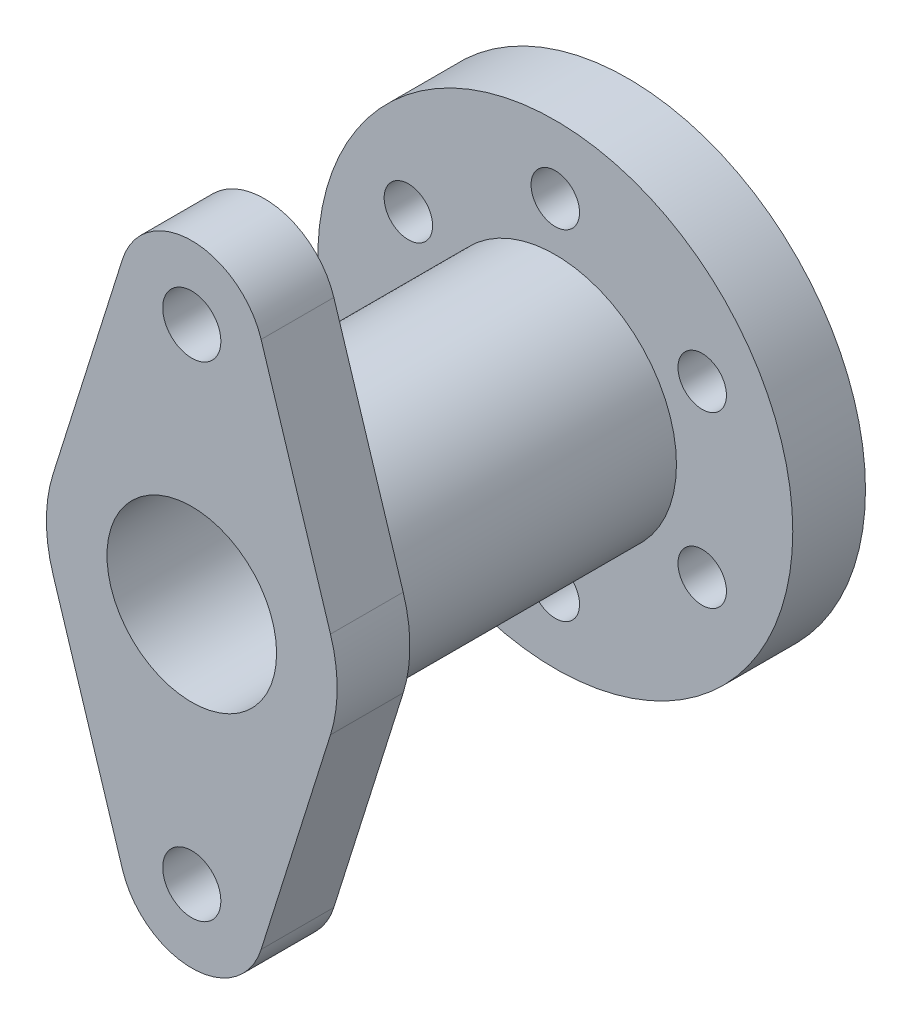
ISO-10303-21;
HEADER;
FILE_DESCRIPTION(('STEP AP214'),'2;1');
FILE_NAME('part.step','',(''),(''),'','','');
FILE_SCHEMA(('AUTOMOTIVE_DESIGN { 1 0 10303 214 1 1 1 1 }'));
ENDSEC;
DATA;
#1=APPLICATION_CONTEXT('core data for automotive mechanical design processes');
#2=APPLICATION_PROTOCOL_DEFINITION('international standard','automotive_design',2000,#1);
#3=PRODUCT_CONTEXT('',#1,'mechanical');
#4=PRODUCT('Part','Part','',(#3));
#5=PRODUCT_RELATED_PRODUCT_CATEGORY('part','',(#4));
#6=PRODUCT_DEFINITION_FORMATION('','',#4);
#7=PRODUCT_DEFINITION_CONTEXT('part definition',#1,'design');
#8=PRODUCT_DEFINITION('design','',#6,#7);
#9=PRODUCT_DEFINITION_SHAPE('','',#8);
#10=(LENGTH_UNIT() NAMED_UNIT(*) SI_UNIT(.MILLI.,.METRE.));
#11=(NAMED_UNIT(*) PLANE_ANGLE_UNIT() SI_UNIT($,.RADIAN.));
#12=(NAMED_UNIT(*) SI_UNIT($,.STERADIAN.) SOLID_ANGLE_UNIT());
#13=UNCERTAINTY_MEASURE_WITH_UNIT(LENGTH_MEASURE(1.E-05),#10,'distance_accuracy_value','');
#14=(GEOMETRIC_REPRESENTATION_CONTEXT(3) GLOBAL_UNCERTAINTY_ASSIGNED_CONTEXT((#13)) GLOBAL_UNIT_ASSIGNED_CONTEXT((#10,
#11,#12)) REPRESENTATION_CONTEXT('',''));
#15=CARTESIAN_POINT('',(0.,0.,0.));
#16=DIRECTION('',(0.,0.,1.));
#17=DIRECTION('',(1.,0.,0.));
#18=AXIS2_PLACEMENT_3D('',#15,#16,#17);
#19=CARTESIAN_POINT('',(0.,0.,60.));
#20=DIRECTION('',(0.,0.,1.));
#21=DIRECTION('',(1.,0.,0.));
#22=AXIS2_PLACEMENT_3D('',#19,#20,#21);
#23=PLANE('',#22);
#24=CARTESIAN_POINT('',(0.,0.,60.));
#25=DIRECTION('',(0.,0.,1.));
#26=DIRECTION('',(1.,0.,0.));
#27=AXIS2_PLACEMENT_3D('',#24,#25,#26);
#28=CIRCLE('',#27,13.);
#29=CARTESIAN_POINT('',(13.,0.,60.));
#30=VERTEX_POINT('',#29);
#31=EDGE_CURVE('E194',#30,#30,#28,.T.);
#32=ORIENTED_EDGE('',*,*,#31,.F.);
#33=EDGE_LOOP('',(#32));
#34=FACE_BOUND('',#33,.T.);
#35=CARTESIAN_POINT('',(0.,0.,60.));
#36=DIRECTION('',(0.,0.,1.));
#37=DIRECTION('',(1.,0.,0.));
#38=AXIS2_PLACEMENT_3D('',#35,#36,#37);
#39=CIRCLE('',#38,17.5);
#40=CARTESIAN_POINT('',(17.5,0.,60.));
#41=VERTEX_POINT('',#40);
#42=EDGE_CURVE('E187',#41,#41,#39,.T.);
#43=ORIENTED_EDGE('',*,*,#42,.T.);
#44=EDGE_LOOP('',(#43));
#45=FACE_BOUND('',#44,.T.);
#46=ADVANCED_FACE('F50',(#34,#45),#23,.T.);
#47=CARTESIAN_POINT('',(0.,0.,15.));
#48=DIRECTION('',(0.,0.,1.));
#49=DIRECTION('',(1.,0.,0.));
#50=AXIS2_PLACEMENT_3D('',#47,#48,#49);
#51=PLANE('',#50);
#52=CARTESIAN_POINT('',(-30.3108891324546,17.4999999999987,15.));
#53=DIRECTION('',(0.,0.,1.));
#54=DIRECTION('',(1.,0.,0.));
#55=AXIS2_PLACEMENT_3D('',#52,#53,#54);
#56=CIRCLE('',#55,5.0000000000015);
#57=CARTESIAN_POINT('',(-25.3108891324531,17.4999999999987,15.));
#58=VERTEX_POINT('',#57);
#59=EDGE_CURVE('E203',#58,#58,#56,.T.);
#60=ORIENTED_EDGE('',*,*,#59,.F.);
#61=EDGE_LOOP('',(#60));
#62=FACE_BOUND('',#61,.T.);
#63=CARTESIAN_POINT('',(2.97142069880137E-12,-35.,15.));
#64=DIRECTION('',(0.,0.,1.));
#65=DIRECTION('',(1.,0.,0.));
#66=AXIS2_PLACEMENT_3D('',#63,#64,#65);
#67=CIRCLE('',#66,5.00000000000308);
#68=CARTESIAN_POINT('',(5.00000000000605,-35.,15.));
#69=VERTEX_POINT('',#68);
#70=EDGE_CURVE('E213',#69,#69,#67,.T.);
#71=ORIENTED_EDGE('',*,*,#70,.F.);
#72=EDGE_LOOP('',(#71));
#73=FACE_BOUND('',#72,.T.);
#74=CARTESIAN_POINT('',(30.3108891324561,17.5000000000013,15.));
#75=DIRECTION('',(0.,0.,1.));
#76=DIRECTION('',(1.,0.,0.));
#77=AXIS2_PLACEMENT_3D('',#74,#75,#76);
#78=CIRCLE('',#77,5.00000000000041);
#79=CARTESIAN_POINT('',(35.3108891324565,17.5000000000013,15.));
#80=VERTEX_POINT('',#79);
#81=EDGE_CURVE('E223',#80,#80,#78,.T.);
#82=ORIENTED_EDGE('',*,*,#81,.F.);
#83=EDGE_LOOP('',(#82));
#84=FACE_BOUND('',#83,.T.);
#85=CARTESIAN_POINT('',(0.,0.,15.));
#86=DIRECTION('',(0.,0.,1.));
#87=DIRECTION('',(1.,0.,0.));
#88=AXIS2_PLACEMENT_3D('',#85,#86,#87);
#89=CIRCLE('',#88,49.);
#90=CARTESIAN_POINT('',(49.,0.,15.));
#91=VERTEX_POINT('',#90);
#92=EDGE_CURVE('E11',#91,#91,#89,.T.);
#93=ORIENTED_EDGE('',*,*,#92,.T.);
#94=EDGE_LOOP('',(#93));
#95=FACE_BOUND('',#94,.T.);
#96=CARTESIAN_POINT('',(0.,35.,15.));
#97=DIRECTION('',(0.,0.,1.));
#98=DIRECTION('',(1.,0.,0.));
#99=AXIS2_PLACEMENT_3D('',#96,#97,#98);
#100=CIRCLE('',#99,5.);
#101=CARTESIAN_POINT('',(5.,35.,15.));
#102=VERTEX_POINT('',#101);
#103=EDGE_CURVE('E233',#102,#102,#100,.T.);
#104=ORIENTED_EDGE('',*,*,#103,.F.);
#105=EDGE_LOOP('',(#104));
#106=FACE_BOUND('',#105,.T.);
#107=CARTESIAN_POINT('',(30.3108891324576,-17.4999999999987,15.));
#108=DIRECTION('',(0.,0.,1.));
#109=DIRECTION('',(1.,0.,0.));
#110=AXIS2_PLACEMENT_3D('',#107,#108,#109);
#111=CIRCLE('',#110,5.00000000000192);
#112=CARTESIAN_POINT('',(35.3108891324595,-17.4999999999987,15.));
#113=VERTEX_POINT('',#112);
#114=EDGE_CURVE('E218',#113,#113,#111,.T.);
#115=ORIENTED_EDGE('',*,*,#114,.F.);
#116=EDGE_LOOP('',(#115));
#117=FACE_BOUND('',#116,.T.);
#118=CARTESIAN_POINT('',(-30.3108891324531,-17.5000000000013,15.));
#119=DIRECTION('',(0.,0.,1.));
#120=DIRECTION('',(1.,0.,0.));
#121=AXIS2_PLACEMENT_3D('',#118,#119,#120);
#122=CIRCLE('',#121,5.00000000000282);
#123=CARTESIAN_POINT('',(-25.3108891324503,-17.5000000000013,15.));
#124=VERTEX_POINT('',#123);
#125=EDGE_CURVE('E210',#124,#124,#122,.T.);
#126=ORIENTED_EDGE('',*,*,#125,.F.);
#127=EDGE_LOOP('',(#126));
#128=FACE_BOUND('',#127,.T.);
#129=CARTESIAN_POINT('',(0.,0.,15.));
#130=DIRECTION('',(0.,0.,1.));
#131=DIRECTION('',(1.,0.,0.));
#132=AXIS2_PLACEMENT_3D('',#129,#130,#131);
#133=CIRCLE('',#132,25.);
#134=CARTESIAN_POINT('',(-25.,0.,15.));
#135=VERTEX_POINT('',#134);
#136=EDGE_CURVE('E197',#135,#135,#133,.T.);
#137=ORIENTED_EDGE('',*,*,#136,.F.);
#138=EDGE_LOOP('',(#137));
#139=FACE_BOUND('',#138,.T.);
#140=ADVANCED_FACE('F248',(#62,#73,#84,#95,#106,#117,#128,#139),#51,.T.);
#141=CARTESIAN_POINT('',(0.,0.,0.));
#142=DIRECTION('',(0.,0.,1.));
#143=DIRECTION('',(1.,0.,0.));
#144=AXIS2_PLACEMENT_3D('',#141,#142,#143);
#145=PLANE('',#144);
#146=CARTESIAN_POINT('',(0.,0.,0.));
#147=DIRECTION('',(0.,0.,1.));
#148=DIRECTION('',(1.,0.,0.));
#149=AXIS2_PLACEMENT_3D('',#146,#147,#148);
#150=CIRCLE('',#149,49.);
#151=CARTESIAN_POINT('',(49.,0.,0.));
#152=VERTEX_POINT('',#151);
#153=EDGE_CURVE('E51',#152,#152,#150,.T.);
#154=ORIENTED_EDGE('',*,*,#153,.F.);
#155=EDGE_LOOP('',(#154));
#156=FACE_BOUND('',#155,.T.);
#157=CARTESIAN_POINT('',(0.,0.,0.));
#158=DIRECTION('',(0.,0.,1.));
#159=DIRECTION('',(1.,0.,0.));
#160=AXIS2_PLACEMENT_3D('',#157,#158,#159);
#161=CIRCLE('',#160,13.);
#162=CARTESIAN_POINT('',(13.,0.,0.));
#163=VERTEX_POINT('',#162);
#164=EDGE_CURVE('E234',#163,#163,#161,.T.);
#165=ORIENTED_EDGE('',*,*,#164,.T.);
#166=EDGE_LOOP('',(#165));
#167=FACE_BOUND('',#166,.T.);
#168=CARTESIAN_POINT('',(0.,35.,0.));
#169=DIRECTION('',(0.,0.,1.));
#170=DIRECTION('',(1.,0.,0.));
#171=AXIS2_PLACEMENT_3D('',#168,#169,#170);
#172=CIRCLE('',#171,5.);
#173=CARTESIAN_POINT('',(5.,35.,0.));
#174=VERTEX_POINT('',#173);
#175=EDGE_CURVE('E227',#174,#174,#172,.T.);
#176=ORIENTED_EDGE('',*,*,#175,.T.);
#177=EDGE_LOOP('',(#176));
#178=FACE_BOUND('',#177,.T.);
#179=CARTESIAN_POINT('',(30.3108891324561,17.5000000000013,0.));
#180=DIRECTION('',(0.,0.,1.));
#181=DIRECTION('',(1.,0.,0.));
#182=AXIS2_PLACEMENT_3D('',#179,#180,#181);
#183=CIRCLE('',#182,5.00000000000041);
#184=CARTESIAN_POINT('',(35.3108891324565,17.5000000000013,0.));
#185=VERTEX_POINT('',#184);
#186=EDGE_CURVE('E225',#185,#185,#183,.T.);
#187=ORIENTED_EDGE('',*,*,#186,.T.);
#188=EDGE_LOOP('',(#187));
#189=FACE_BOUND('',#188,.T.);
#190=CARTESIAN_POINT('',(30.3108891324576,-17.4999999999987,0.));
#191=DIRECTION('',(0.,0.,1.));
#192=DIRECTION('',(1.,0.,0.));
#193=AXIS2_PLACEMENT_3D('',#190,#191,#192);
#194=CIRCLE('',#193,5.00000000000192);
#195=CARTESIAN_POINT('',(35.3108891324595,-17.4999999999987,0.));
#196=VERTEX_POINT('',#195);
#197=EDGE_CURVE('E216',#196,#196,#194,.T.);
#198=ORIENTED_EDGE('',*,*,#197,.T.);
#199=EDGE_LOOP('',(#198));
#200=FACE_BOUND('',#199,.T.);
#201=CARTESIAN_POINT('',(2.97142069880137E-12,-35.,0.));
#202=DIRECTION('',(0.,0.,1.));
#203=DIRECTION('',(1.,0.,0.));
#204=AXIS2_PLACEMENT_3D('',#201,#202,#203);
#205=CIRCLE('',#204,5.00000000000308);
#206=CARTESIAN_POINT('',(5.00000000000605,-35.,0.));
#207=VERTEX_POINT('',#206);
#208=EDGE_CURVE('E209',#207,#207,#205,.T.);
#209=ORIENTED_EDGE('',*,*,#208,.T.);
#210=EDGE_LOOP('',(#209));
#211=FACE_BOUND('',#210,.T.);
#212=CARTESIAN_POINT('',(-30.3108891324531,-17.5000000000013,0.));
#213=DIRECTION('',(0.,0.,1.));
#214=DIRECTION('',(1.,0.,0.));
#215=AXIS2_PLACEMENT_3D('',#212,#213,#214);
#216=CIRCLE('',#215,5.00000000000282);
#217=CARTESIAN_POINT('',(-25.3108891324503,-17.5000000000013,0.));
#218=VERTEX_POINT('',#217);
#219=EDGE_CURVE('E204',#218,#218,#216,.T.);
#220=ORIENTED_EDGE('',*,*,#219,.T.);
#221=EDGE_LOOP('',(#220));
#222=FACE_BOUND('',#221,.T.);
#223=CARTESIAN_POINT('',(-30.3108891324546,17.4999999999987,0.));
#224=DIRECTION('',(0.,0.,1.));
#225=DIRECTION('',(1.,0.,0.));
#226=AXIS2_PLACEMENT_3D('',#223,#224,#225);
#227=CIRCLE('',#226,5.0000000000015);
#228=CARTESIAN_POINT('',(-25.3108891324531,17.4999999999987,0.));
#229=VERTEX_POINT('',#228);
#230=EDGE_CURVE('E199',#229,#229,#227,.T.);
#231=ORIENTED_EDGE('',*,*,#230,.T.);
#232=EDGE_LOOP('',(#231));
#233=FACE_BOUND('',#232,.T.);
#234=ADVANCED_FACE('F243',(#156,#167,#178,#189,#200,#211,#222,#233),#145,.F.);
#235=CARTESIAN_POINT('',(0.,0.,15.));
#236=DIRECTION('',(0.,0.,-1.));
#237=DIRECTION('',(-1.,0.,0.));
#238=AXIS2_PLACEMENT_3D('',#235,#236,#237);
#239=CYLINDRICAL_SURFACE('',#238,49.);
#240=ORIENTED_EDGE('',*,*,#92,.F.);
#241=EDGE_LOOP('',(#240));
#242=FACE_BOUND('',#241,.T.);
#243=ORIENTED_EDGE('',*,*,#153,.T.);
#244=EDGE_LOOP('',(#243));
#245=FACE_BOUND('',#244,.T.);
#246=ADVANCED_FACE('F47',(#242,#245),#239,.T.);
#247=CARTESIAN_POINT('',(0.,0.,15.));
#248=DIRECTION('',(0.,0.,-1.));
#249=DIRECTION('',(-1.,0.,0.));
#250=AXIS2_PLACEMENT_3D('',#247,#248,#249);
#251=CYLINDRICAL_SURFACE('',#250,13.);
#252=ORIENTED_EDGE('',*,*,#164,.F.);
#253=EDGE_LOOP('',(#252));
#254=FACE_BOUND('',#253,.T.);
#255=ORIENTED_EDGE('',*,*,#31,.T.);
#256=EDGE_LOOP('',(#255));
#257=FACE_BOUND('',#256,.T.);
#258=ADVANCED_FACE('F556',(#254,#257),#251,.F.);
#259=CARTESIAN_POINT('',(0.,35.,15.));
#260=DIRECTION('',(0.,0.,-1.));
#261=DIRECTION('',(-1.,0.,0.));
#262=AXIS2_PLACEMENT_3D('',#259,#260,#261);
#263=CYLINDRICAL_SURFACE('',#262,5.);
#264=ORIENTED_EDGE('',*,*,#103,.T.);
#265=EDGE_LOOP('',(#264));
#266=FACE_BOUND('',#265,.T.);
#267=ORIENTED_EDGE('',*,*,#175,.F.);
#268=EDGE_LOOP('',(#267));
#269=FACE_BOUND('',#268,.T.);
#270=ADVANCED_FACE('F546',(#266,#269),#263,.F.);
#271=CARTESIAN_POINT('',(30.3108891324561,17.5000000000013,15.));
#272=DIRECTION('',(0.,0.,-1.));
#273=DIRECTION('',(-1.,0.,0.));
#274=AXIS2_PLACEMENT_3D('',#271,#272,#273);
#275=CYLINDRICAL_SURFACE('',#274,5.00000000000041);
#276=ORIENTED_EDGE('',*,*,#81,.T.);
#277=EDGE_LOOP('',(#276));
#278=FACE_BOUND('',#277,.T.);
#279=ORIENTED_EDGE('',*,*,#186,.F.);
#280=EDGE_LOOP('',(#279));
#281=FACE_BOUND('',#280,.T.);
#282=ADVANCED_FACE('F536',(#278,#281),#275,.F.);
#283=CARTESIAN_POINT('',(30.3108891324576,-17.4999999999987,15.));
#284=DIRECTION('',(0.,0.,-1.));
#285=DIRECTION('',(-1.,0.,0.));
#286=AXIS2_PLACEMENT_3D('',#283,#284,#285);
#287=CYLINDRICAL_SURFACE('',#286,5.00000000000192);
#288=ORIENTED_EDGE('',*,*,#114,.T.);
#289=EDGE_LOOP('',(#288));
#290=FACE_BOUND('',#289,.T.);
#291=ORIENTED_EDGE('',*,*,#197,.F.);
#292=EDGE_LOOP('',(#291));
#293=FACE_BOUND('',#292,.T.);
#294=ADVANCED_FACE('F528',(#290,#293),#287,.F.);
#295=CARTESIAN_POINT('',(2.97142069880137E-12,-35.,15.));
#296=DIRECTION('',(0.,0.,-1.));
#297=DIRECTION('',(-1.,0.,0.));
#298=AXIS2_PLACEMENT_3D('',#295,#296,#297);
#299=CYLINDRICAL_SURFACE('',#298,5.00000000000308);
#300=ORIENTED_EDGE('',*,*,#70,.T.);
#301=EDGE_LOOP('',(#300));
#302=FACE_BOUND('',#301,.T.);
#303=ORIENTED_EDGE('',*,*,#208,.F.);
#304=EDGE_LOOP('',(#303));
#305=FACE_BOUND('',#304,.T.);
#306=ADVANCED_FACE('F272',(#302,#305),#299,.F.);
#307=CARTESIAN_POINT('',(-30.3108891324531,-17.5000000000013,15.));
#308=DIRECTION('',(0.,0.,-1.));
#309=DIRECTION('',(-1.,0.,0.));
#310=AXIS2_PLACEMENT_3D('',#307,#308,#309);
#311=CYLINDRICAL_SURFACE('',#310,5.00000000000282);
#312=ORIENTED_EDGE('',*,*,#125,.T.);
#313=EDGE_LOOP('',(#312));
#314=FACE_BOUND('',#313,.T.);
#315=ORIENTED_EDGE('',*,*,#219,.F.);
#316=EDGE_LOOP('',(#315));
#317=FACE_BOUND('',#316,.T.);
#318=ADVANCED_FACE('F263',(#314,#317),#311,.F.);
#319=CARTESIAN_POINT('',(-30.3108891324546,17.4999999999987,15.));
#320=DIRECTION('',(0.,0.,-1.));
#321=DIRECTION('',(-1.,0.,0.));
#322=AXIS2_PLACEMENT_3D('',#319,#320,#321);
#323=CYLINDRICAL_SURFACE('',#322,5.0000000000015);
#324=ORIENTED_EDGE('',*,*,#59,.T.);
#325=EDGE_LOOP('',(#324));
#326=FACE_BOUND('',#325,.T.);
#327=ORIENTED_EDGE('',*,*,#230,.F.);
#328=EDGE_LOOP('',(#327));
#329=FACE_BOUND('',#328,.T.);
#330=ADVANCED_FACE('F257',(#326,#329),#323,.F.);
#331=CARTESIAN_POINT('',(0.,0.,60.));
#332=DIRECTION('',(0.,0.,-1.));
#333=DIRECTION('',(-1.,0.,0.));
#334=AXIS2_PLACEMENT_3D('',#331,#332,#333);
#335=CYLINDRICAL_SURFACE('',#334,25.);
#336=CARTESIAN_POINT('',(0.,0.,75.));
#337=DIRECTION('',(0.,0.,1.));
#338=DIRECTION('',(1.,0.,0.));
#339=AXIS2_PLACEMENT_3D('',#336,#337,#338);
#340=CIRCLE('',#339,25.);
#341=CARTESIAN_POINT('',(-25.,0.,75.));
#342=VERTEX_POINT('',#341);
#343=EDGE_CURVE('E193',#342,#342,#340,.T.);
#344=CARTESIAN_POINT('',(-25.,0.,15.));
#345=CARTESIAN_POINT('',(-25.,0.,15.625));
#346=CARTESIAN_POINT('',(-25.,0.,16.25));
#347=CARTESIAN_POINT('',(-25.,0.,17.5));
#348=CARTESIAN_POINT('',(-25.,0.,18.125));
#349=CARTESIAN_POINT('',(-25.,0.,19.375));
#350=CARTESIAN_POINT('',(-25.,0.,20.));
#351=CARTESIAN_POINT('',(-25.,0.,21.25));
#352=CARTESIAN_POINT('',(-25.,0.,21.875));
#353=CARTESIAN_POINT('',(-25.,0.,23.125));
#354=CARTESIAN_POINT('',(-25.,0.,23.75));
#355=CARTESIAN_POINT('',(-25.,0.,25.));
#356=CARTESIAN_POINT('',(-25.,0.,25.625));
#357=CARTESIAN_POINT('',(-25.,0.,26.875));
#358=CARTESIAN_POINT('',(-25.,0.,27.5));
#359=CARTESIAN_POINT('',(-25.,0.,28.75));
#360=CARTESIAN_POINT('',(-25.,0.,29.375));
#361=CARTESIAN_POINT('',(-25.,0.,30.625));
#362=CARTESIAN_POINT('',(-25.,0.,31.25));
#363=CARTESIAN_POINT('',(-25.,0.,32.5));
#364=CARTESIAN_POINT('',(-25.,0.,33.125));
#365=CARTESIAN_POINT('',(-25.,0.,34.375));
#366=CARTESIAN_POINT('',(-25.,0.,35.));
#367=CARTESIAN_POINT('',(-25.,0.,36.25));
#368=CARTESIAN_POINT('',(-25.,0.,36.875));
#369=CARTESIAN_POINT('',(-25.,0.,38.125));
#370=CARTESIAN_POINT('',(-25.,0.,38.75));
#371=CARTESIAN_POINT('',(-25.,0.,40.));
#372=CARTESIAN_POINT('',(-25.,0.,40.625));
#373=CARTESIAN_POINT('',(-25.,0.,41.875));
#374=CARTESIAN_POINT('',(-25.,0.,42.5));
#375=CARTESIAN_POINT('',(-25.,0.,43.75));
#376=CARTESIAN_POINT('',(-25.,0.,44.375));
#377=CARTESIAN_POINT('',(-25.,0.,45.625));
#378=CARTESIAN_POINT('',(-25.,0.,46.25));
#379=CARTESIAN_POINT('',(-25.,0.,47.5));
#380=CARTESIAN_POINT('',(-25.,0.,48.125));
#381=CARTESIAN_POINT('',(-25.,0.,49.375));
#382=CARTESIAN_POINT('',(-25.,0.,50.));
#383=CARTESIAN_POINT('',(-25.,0.,51.25));
#384=CARTESIAN_POINT('',(-25.,0.,51.875));
#385=CARTESIAN_POINT('',(-25.,0.,53.125));
#386=CARTESIAN_POINT('',(-25.,0.,53.75));
#387=CARTESIAN_POINT('',(-25.,0.,55.));
#388=CARTESIAN_POINT('',(-25.,0.,55.625));
#389=CARTESIAN_POINT('',(-25.,0.,56.875));
#390=CARTESIAN_POINT('',(-25.,0.,57.5));
#391=CARTESIAN_POINT('',(-25.,0.,58.75));
#392=CARTESIAN_POINT('',(-25.,0.,59.375));
#393=CARTESIAN_POINT('',(-25.,0.,60.625));
#394=CARTESIAN_POINT('',(-25.,0.,61.25));
#395=CARTESIAN_POINT('',(-25.,0.,62.5));
#396=CARTESIAN_POINT('',(-25.,0.,63.125));
#397=CARTESIAN_POINT('',(-25.,0.,64.375));
#398=CARTESIAN_POINT('',(-25.,0.,65.));
#399=CARTESIAN_POINT('',(-25.,0.,66.25));
#400=CARTESIAN_POINT('',(-25.,0.,66.875));
#401=CARTESIAN_POINT('',(-25.,0.,68.125));
#402=CARTESIAN_POINT('',(-25.,0.,68.75));
#403=CARTESIAN_POINT('',(-25.,0.,70.));
#404=CARTESIAN_POINT('',(-25.,0.,70.625));
#405=CARTESIAN_POINT('',(-25.,0.,71.875));
#406=CARTESIAN_POINT('',(-25.,0.,72.5));
#407=CARTESIAN_POINT('',(-25.,0.,73.75));
#408=CARTESIAN_POINT('',(-25.,0.,74.375));
#409=CARTESIAN_POINT('',(-25.,0.,75.));
#410=B_SPLINE_CURVE_WITH_KNOTS('',3,(#344,#345,#346,#347,#348,#349,#350,#351,#352,#353,#354,
#355,#356,#357,#358,#359,#360,#361,#362,#363,#364,#365,#366,#367,#368,#369,#370,#371,#372,#373,
#374,#375,#376,#377,#378,#379,#380,#381,#382,#383,#384,#385,#386,#387,#388,#389,#390,#391,#392,
#393,#394,#395,#396,#397,#398,#399,#400,#401,#402,#403,#404,#405,#406,#407,#408,#409),
.UNSPECIFIED.,.F.,.F.,(4,2,2,2,2,2,2,2,2,2,2,2,2,2,2,2,2,2,2,2,2,2,2,2,2,2,2,2,2,2,2,2,4),(0.,
1.875,3.75,5.62500000000001,7.5,9.375,11.25,13.125,15.,16.875,18.75,20.625,22.5,24.375,26.25,
28.125,30.,31.875,33.75,35.625,37.5,39.375,41.25,43.125,45.,46.875,48.75,50.625,52.5,54.375,
56.25,58.125,60.),.UNSPECIFIED.);
#411=EDGE_CURVE('BSEAM265',#135,#342,#410,.T.);
#412=ORIENTED_EDGE('',*,*,#136,.T.);
#413=ORIENTED_EDGE('',*,*,#343,.F.);
#414=ORIENTED_EDGE('',*,*,#411,.T.);
#415=ORIENTED_EDGE('',*,*,#411,.F.);
#416=EDGE_LOOP('',(#412,#414,#413,#415));
#417=FACE_BOUND('',#416,.T.);
#418=ADVANCED_FACE('F265',(#417),#335,.T.);
#419=CARTESIAN_POINT('',(0.,0.,75.));
#420=DIRECTION('',(0.,0.,-1.));
#421=DIRECTION('',(-1.,0.,0.));
#422=AXIS2_PLACEMENT_3D('',#419,#420,#421);
#423=CYLINDRICAL_SURFACE('',#422,17.5);
#424=ORIENTED_EDGE('',*,*,#42,.F.);
#425=EDGE_LOOP('',(#424));
#426=FACE_BOUND('',#425,.T.);
#427=CARTESIAN_POINT('',(0.,0.,90.));
#428=DIRECTION('',(0.,0.,1.));
#429=DIRECTION('',(1.,0.,0.));
#430=AXIS2_PLACEMENT_3D('',#427,#428,#429);
#431=CIRCLE('',#430,17.5);
#432=CARTESIAN_POINT('',(17.5,0.,90.));
#433=VERTEX_POINT('',#432);
#434=EDGE_CURVE('E149',#433,#433,#431,.F.);
#435=ORIENTED_EDGE('',*,*,#434,.F.);
#436=EDGE_LOOP('',(#435));
#437=FACE_BOUND('',#436,.T.);
#438=ADVANCED_FACE('F269',(#426,#437),#423,.F.);
#439=CARTESIAN_POINT('',(28.6181760425084,-9.,90.));
#440=DIRECTION('',(0.953939201416946,-0.3,0.));
#441=DIRECTION('',(0.3,0.953939201416946,0.));
#442=AXIS2_PLACEMENT_3D('',#439,#440,#441);
#443=PLANE('',#442);
#444=DIRECTION('',(-0.3,-0.953939201416946,0.));
#445=VECTOR('',#444,1.);
#446=CARTESIAN_POINT('',(28.6181760425084,-9.,75.));
#447=LINE('',#446,#445);
#448=CARTESIAN_POINT('',(28.6181760425084,-9.,75.));
#449=VERTEX_POINT('',#448);
#450=CARTESIAN_POINT('',(14.3090880212542,-54.5,75.));
#451=VERTEX_POINT('',#450);
#452=EDGE_CURVE('E155',#449,#451,#447,.T.);
#453=ORIENTED_EDGE('',*,*,#452,.F.);
#454=DIRECTION('',(0.,0.,-1.));
#455=VECTOR('',#454,1.);
#456=CARTESIAN_POINT('',(28.6181760425084,-9.,90.));
#457=LINE('',#456,#455);
#458=CARTESIAN_POINT('',(28.6181760425084,-9.,90.));
#459=VERTEX_POINT('',#458);
#460=EDGE_CURVE('E104',#459,#449,#457,.T.);
#461=ORIENTED_EDGE('',*,*,#460,.F.);
#462=DIRECTION('',(-0.3,-0.953939201416946,0.));
#463=VECTOR('',#462,1.);
#464=CARTESIAN_POINT('',(28.6181760425084,-9.,90.));
#465=LINE('',#464,#463);
#466=CARTESIAN_POINT('',(14.3090880212542,-54.5,90.));
#467=VERTEX_POINT('',#466);
#468=EDGE_CURVE('E174',#459,#467,#465,.T.);
#469=ORIENTED_EDGE('',*,*,#468,.T.);
#470=DIRECTION('',(0.,0.,-1.));
#471=VECTOR('',#470,1.);
#472=CARTESIAN_POINT('',(14.3090880212542,-54.5,90.));
#473=LINE('',#472,#471);
#474=EDGE_CURVE('E99',#467,#451,#473,.T.);
#475=ORIENTED_EDGE('',*,*,#474,.T.);
#476=EDGE_LOOP('',(#453,#461,#469,#475));
#477=FACE_BOUND('',#476,.T.);
#478=ADVANCED_FACE('F287',(#477),#443,.T.);
#479=CARTESIAN_POINT('',(0.,0.,90.));
#480=DIRECTION('',(0.,0.,-1.));
#481=DIRECTION('',(-1.,0.,0.));
#482=AXIS2_PLACEMENT_3D('',#479,#480,#481);
#483=CYLINDRICAL_SURFACE('',#482,30.);
#484=CARTESIAN_POINT('',(0.,0.,75.));
#485=DIRECTION('',(0.,0.,1.));
#486=DIRECTION('',(1.,0.,0.));
#487=AXIS2_PLACEMENT_3D('',#484,#485,#486);
#488=CIRCLE('',#487,30.);
#489=CARTESIAN_POINT('',(28.6181760425084,9.,75.));
#490=VERTEX_POINT('',#489);
#491=EDGE_CURVE('E154',#449,#490,#488,.T.);
#492=ORIENTED_EDGE('',*,*,#491,.T.);
#493=DIRECTION('',(0.,0.,-1.));
#494=VECTOR('',#493,1.);
#495=CARTESIAN_POINT('',(28.6181760425084,9.,90.));
#496=LINE('',#495,#494);
#497=CARTESIAN_POINT('',(28.6181760425084,9.,90.));
#498=VERTEX_POINT('',#497);
#499=EDGE_CURVE('E184',#498,#490,#496,.T.);
#500=ORIENTED_EDGE('',*,*,#499,.F.);
#501=CARTESIAN_POINT('',(0.,0.,90.));
#502=DIRECTION('',(0.,0.,1.));
#503=DIRECTION('',(1.,0.,0.));
#504=AXIS2_PLACEMENT_3D('',#501,#502,#503);
#505=CIRCLE('',#504,30.);
#506=EDGE_CURVE('E688',#459,#498,#505,.T.);
#507=ORIENTED_EDGE('',*,*,#506,.F.);
#508=ORIENTED_EDGE('',*,*,#460,.T.);
#509=EDGE_LOOP('',(#492,#500,#507,#508));
#510=FACE_BOUND('',#509,.T.);
#511=ADVANCED_FACE('F294',(#510),#483,.T.);
#512=CARTESIAN_POINT('',(28.6181760425084,9.00000000000003,90.));
#513=DIRECTION('',(-0.953939201416945,-0.300000000000001,0.));
#514=DIRECTION('',(0.300000000000001,-0.953939201416945,0.));
#515=AXIS2_PLACEMENT_3D('',#512,#513,#514);
#516=PLANE('',#515);
#517=DIRECTION('',(-0.300000000000001,0.953939201416945,0.));
#518=VECTOR('',#517,1.);
#519=CARTESIAN_POINT('',(28.6181760425084,9.00000000000003,75.));
#520=LINE('',#519,#518);
#521=CARTESIAN_POINT('',(14.3090880212542,54.5,75.));
#522=VERTEX_POINT('',#521);
#523=EDGE_CURVE('E160',#490,#522,#520,.T.);
#524=ORIENTED_EDGE('',*,*,#523,.T.);
#525=DIRECTION('',(0.,0.,-1.));
#526=VECTOR('',#525,1.);
#527=CARTESIAN_POINT('',(14.3090880212542,54.5,90.));
#528=LINE('',#527,#526);
#529=CARTESIAN_POINT('',(14.3090880212542,54.5,90.));
#530=VERTEX_POINT('',#529);
#531=EDGE_CURVE('E182',#530,#522,#528,.T.);
#532=ORIENTED_EDGE('',*,*,#531,.F.);
#533=DIRECTION('',(-0.300000000000001,0.953939201416945,0.));
#534=VECTOR('',#533,1.);
#535=CARTESIAN_POINT('',(28.6181760425084,9.00000000000003,90.));
#536=LINE('',#535,#534);
#537=EDGE_CURVE('E682',#498,#530,#536,.T.);
#538=ORIENTED_EDGE('',*,*,#537,.F.);
#539=ORIENTED_EDGE('',*,*,#499,.T.);
#540=EDGE_LOOP('',(#524,#532,#538,#539));
#541=FACE_BOUND('',#540,.T.);
#542=ADVANCED_FACE('F300',(#541),#516,.F.);
#543=CARTESIAN_POINT('',(0.,50.,90.));
#544=DIRECTION('',(0.,0.,-1.));
#545=DIRECTION('',(-1.,0.,0.));
#546=AXIS2_PLACEMENT_3D('',#543,#544,#545);
#547=CYLINDRICAL_SURFACE('',#546,15.);
#548=CARTESIAN_POINT('',(0.,50.,75.));
#549=DIRECTION('',(0.,0.,1.));
#550=DIRECTION('',(1.,0.,0.));
#551=AXIS2_PLACEMENT_3D('',#548,#549,#550);
#552=CIRCLE('',#551,15.);
#553=CARTESIAN_POINT('',(-14.3090880212542,54.5,75.));
#554=VERTEX_POINT('',#553);
#555=EDGE_CURVE('E157',#522,#554,#552,.T.);
#556=ORIENTED_EDGE('',*,*,#555,.T.);
#557=DIRECTION('',(0.,0.,-1.));
#558=VECTOR('',#557,1.);
#559=CARTESIAN_POINT('',(-14.3090880212542,54.5,90.));
#560=LINE('',#559,#558);
#561=CARTESIAN_POINT('',(-14.3090880212542,54.5,90.));
#562=VERTEX_POINT('',#561);
#563=EDGE_CURVE('E179',#562,#554,#560,.T.);
#564=ORIENTED_EDGE('',*,*,#563,.F.);
#565=CARTESIAN_POINT('',(0.,50.,90.));
#566=DIRECTION('',(0.,0.,1.));
#567=DIRECTION('',(1.,0.,0.));
#568=AXIS2_PLACEMENT_3D('',#565,#566,#567);
#569=CIRCLE('',#568,15.);
#570=EDGE_CURVE('E684',#530,#562,#569,.T.);
#571=ORIENTED_EDGE('',*,*,#570,.F.);
#572=ORIENTED_EDGE('',*,*,#531,.T.);
#573=EDGE_LOOP('',(#556,#564,#571,#572));
#574=FACE_BOUND('',#573,.T.);
#575=ADVANCED_FACE('F303',(#574),#547,.T.);
#576=CARTESIAN_POINT('',(-28.6181760425084,9.,90.));
#577=DIRECTION('',(-0.953939201416946,0.3,0.));
#578=DIRECTION('',(-0.3,-0.953939201416946,0.));
#579=AXIS2_PLACEMENT_3D('',#576,#577,#578);
#580=PLANE('',#579);
#581=DIRECTION('',(0.3,0.953939201416946,0.));
#582=VECTOR('',#581,1.);
#583=CARTESIAN_POINT('',(-28.6181760425084,9.,75.));
#584=LINE('',#583,#582);
#585=CARTESIAN_POINT('',(-28.6181760425084,9.,75.));
#586=VERTEX_POINT('',#585);
#587=EDGE_CURVE('E165',#586,#554,#584,.T.);
#588=ORIENTED_EDGE('',*,*,#587,.F.);
#589=DIRECTION('',(0.,0.,-1.));
#590=VECTOR('',#589,1.);
#591=CARTESIAN_POINT('',(-28.6181760425084,9.,90.));
#592=LINE('',#591,#590);
#593=CARTESIAN_POINT('',(-28.6181760425084,9.,90.));
#594=VERTEX_POINT('',#593);
#595=EDGE_CURVE('E134',#594,#586,#592,.T.);
#596=ORIENTED_EDGE('',*,*,#595,.F.);
#597=DIRECTION('',(0.3,0.953939201416946,0.));
#598=VECTOR('',#597,1.);
#599=CARTESIAN_POINT('',(-28.6181760425084,9.,90.));
#600=LINE('',#599,#598);
#601=EDGE_CURVE('E126',#594,#562,#600,.T.);
#602=ORIENTED_EDGE('',*,*,#601,.T.);
#603=ORIENTED_EDGE('',*,*,#563,.T.);
#604=EDGE_LOOP('',(#588,#596,#602,#603));
#605=FACE_BOUND('',#604,.T.);
#606=ADVANCED_FACE('F302',(#605),#580,.T.);
#607=CARTESIAN_POINT('',(0.,0.,90.));
#608=DIRECTION('',(0.,0.,-1.));
#609=DIRECTION('',(-1.,0.,0.));
#610=AXIS2_PLACEMENT_3D('',#607,#608,#609);
#611=CYLINDRICAL_SURFACE('',#610,30.);
#612=CARTESIAN_POINT('',(0.,0.,75.));
#613=DIRECTION('',(0.,0.,1.));
#614=DIRECTION('',(1.,0.,0.));
#615=AXIS2_PLACEMENT_3D('',#612,#613,#614);
#616=CIRCLE('',#615,30.);
#617=CARTESIAN_POINT('',(-28.6181760425084,-8.99999999999999,75.));
#618=VERTEX_POINT('',#617);
#619=EDGE_CURVE('E133',#586,#618,#616,.T.);
#620=ORIENTED_EDGE('',*,*,#619,.T.);
#621=DIRECTION('',(0.,0.,-1.));
#622=VECTOR('',#621,1.);
#623=CARTESIAN_POINT('',(-28.6181760425084,-8.99999999999999,90.));
#624=LINE('',#623,#622);
#625=CARTESIAN_POINT('',(-28.6181760425084,-8.99999999999999,90.));
#626=VERTEX_POINT('',#625);
#627=EDGE_CURVE('E131',#626,#618,#624,.T.);
#628=ORIENTED_EDGE('',*,*,#627,.F.);
#629=CARTESIAN_POINT('',(0.,0.,90.));
#630=DIRECTION('',(0.,0.,1.));
#631=DIRECTION('',(1.,0.,0.));
#632=AXIS2_PLACEMENT_3D('',#629,#630,#631);
#633=CIRCLE('',#632,30.);
#634=EDGE_CURVE('E123',#594,#626,#633,.T.);
#635=ORIENTED_EDGE('',*,*,#634,.F.);
#636=ORIENTED_EDGE('',*,*,#595,.T.);
#637=EDGE_LOOP('',(#620,#628,#635,#636));
#638=FACE_BOUND('',#637,.T.);
#639=ADVANCED_FACE('F135',(#638),#611,.T.);
#640=CARTESIAN_POINT('',(-28.6181760425084,-8.99999999999998,90.));
#641=DIRECTION('',(0.953939201416946,0.299999999999999,0.));
#642=DIRECTION('',(-0.299999999999999,0.953939201416946,0.));
#643=AXIS2_PLACEMENT_3D('',#640,#641,#642);
#644=PLANE('',#643);
#645=DIRECTION('',(0.299999999999999,-0.953939201416946,0.));
#646=VECTOR('',#645,1.);
#647=CARTESIAN_POINT('',(-28.6181760425084,-8.99999999999998,75.));
#648=LINE('',#647,#646);
#649=CARTESIAN_POINT('',(-14.3090880212542,-54.5,75.));
#650=VERTEX_POINT('',#649);
#651=EDGE_CURVE('E91',#618,#650,#648,.T.);
#652=ORIENTED_EDGE('',*,*,#651,.T.);
#653=DIRECTION('',(0.,0.,-1.));
#654=VECTOR('',#653,1.);
#655=CARTESIAN_POINT('',(-14.3090880212542,-54.5,90.));
#656=LINE('',#655,#654);
#657=CARTESIAN_POINT('',(-14.3090880212542,-54.5,90.));
#658=VERTEX_POINT('',#657);
#659=EDGE_CURVE('E138',#658,#650,#656,.T.);
#660=ORIENTED_EDGE('',*,*,#659,.F.);
#661=DIRECTION('',(0.299999999999999,-0.953939201416946,0.));
#662=VECTOR('',#661,1.);
#663=CARTESIAN_POINT('',(-28.6181760425084,-8.99999999999998,90.));
#664=LINE('',#663,#662);
#665=EDGE_CURVE('E127',#626,#658,#664,.T.);
#666=ORIENTED_EDGE('',*,*,#665,.F.);
#667=ORIENTED_EDGE('',*,*,#627,.T.);
#668=EDGE_LOOP('',(#652,#660,#666,#667));
#669=FACE_BOUND('',#668,.T.);
#670=ADVANCED_FACE('F136',(#669),#644,.F.);
#671=CARTESIAN_POINT('',(0.,50.,90.));
#672=DIRECTION('',(0.,0.,-1.));
#673=DIRECTION('',(-1.,0.,0.));
#674=AXIS2_PLACEMENT_3D('',#671,#672,#673);
#675=CYLINDRICAL_SURFACE('',#674,6.);
#676=CARTESIAN_POINT('',(0.,50.,90.));
#677=DIRECTION('',(0.,0.,1.));
#678=DIRECTION('',(1.,0.,0.));
#679=AXIS2_PLACEMENT_3D('',#676,#677,#678);
#680=CIRCLE('',#679,6.);
#681=CARTESIAN_POINT('',(6.,50.,90.));
#682=VERTEX_POINT('',#681);
#683=EDGE_CURVE('E148',#682,#682,#680,.T.);
#684=ORIENTED_EDGE('',*,*,#683,.T.);
#685=EDGE_LOOP('',(#684));
#686=FACE_BOUND('',#685,.T.);
#687=CARTESIAN_POINT('',(0.,50.,75.));
#688=DIRECTION('',(0.,0.,1.));
#689=DIRECTION('',(1.,0.,0.));
#690=AXIS2_PLACEMENT_3D('',#687,#688,#689);
#691=CIRCLE('',#690,6.);
#692=CARTESIAN_POINT('',(6.,50.,75.));
#693=VERTEX_POINT('',#692);
#694=EDGE_CURVE('E175',#693,#693,#691,.T.);
#695=ORIENTED_EDGE('',*,*,#694,.F.);
#696=EDGE_LOOP('',(#695));
#697=FACE_BOUND('',#696,.T.);
#698=ADVANCED_FACE('F314',(#686,#697),#675,.F.);
#699=CARTESIAN_POINT('',(0.,-50.,90.));
#700=DIRECTION('',(0.,0.,-1.));
#701=DIRECTION('',(-1.,0.,0.));
#702=AXIS2_PLACEMENT_3D('',#699,#700,#701);
#703=CYLINDRICAL_SURFACE('',#702,6.);
#704=CARTESIAN_POINT('',(0.,-50.,90.));
#705=DIRECTION('',(0.,0.,1.));
#706=DIRECTION('',(1.,0.,0.));
#707=AXIS2_PLACEMENT_3D('',#704,#705,#706);
#708=CIRCLE('',#707,6.);
#709=CARTESIAN_POINT('',(6.,-50.,90.));
#710=VERTEX_POINT('',#709);
#711=EDGE_CURVE('E137',#710,#710,#708,.T.);
#712=ORIENTED_EDGE('',*,*,#711,.T.);
#713=EDGE_LOOP('',(#712));
#714=FACE_BOUND('',#713,.T.);
#715=CARTESIAN_POINT('',(0.,-50.,75.));
#716=DIRECTION('',(0.,0.,1.));
#717=DIRECTION('',(1.,0.,0.));
#718=AXIS2_PLACEMENT_3D('',#715,#716,#717);
#719=CIRCLE('',#718,6.);
#720=CARTESIAN_POINT('',(6.,-50.,75.));
#721=VERTEX_POINT('',#720);
#722=EDGE_CURVE('E166',#721,#721,#719,.T.);
#723=ORIENTED_EDGE('',*,*,#722,.F.);
#724=EDGE_LOOP('',(#723));
#725=FACE_BOUND('',#724,.T.);
#726=ADVANCED_FACE('F318',(#714,#725),#703,.F.);
#727=CARTESIAN_POINT('',(0.,-50.,90.));
#728=DIRECTION('',(0.,0.,-1.));
#729=DIRECTION('',(-1.,0.,0.));
#730=AXIS2_PLACEMENT_3D('',#727,#728,#729);
#731=CYLINDRICAL_SURFACE('',#730,15.);
#732=CARTESIAN_POINT('',(0.,-50.,75.));
#733=DIRECTION('',(0.,0.,1.));
#734=DIRECTION('',(1.,0.,0.));
#735=AXIS2_PLACEMENT_3D('',#732,#733,#734);
#736=CIRCLE('',#735,15.);
#737=EDGE_CURVE('E170',#650,#451,#736,.T.);
#738=ORIENTED_EDGE('',*,*,#737,.T.);
#739=ORIENTED_EDGE('',*,*,#474,.F.);
#740=CARTESIAN_POINT('',(0.,-50.,90.));
#741=DIRECTION('',(0.,0.,1.));
#742=DIRECTION('',(1.,0.,0.));
#743=AXIS2_PLACEMENT_3D('',#740,#741,#742);
#744=CIRCLE('',#743,15.);
#745=EDGE_CURVE('E63',#658,#467,#744,.T.);
#746=ORIENTED_EDGE('',*,*,#745,.F.);
#747=ORIENTED_EDGE('',*,*,#659,.T.);
#748=EDGE_LOOP('',(#738,#739,#746,#747));
#749=FACE_BOUND('',#748,.T.);
#750=ADVANCED_FACE('F312',(#749),#731,.T.);
#751=CARTESIAN_POINT('',(0.,0.,90.));
#752=DIRECTION('',(0.,0.,1.));
#753=DIRECTION('',(1.,0.,0.));
#754=AXIS2_PLACEMENT_3D('',#751,#752,#753);
#755=PLANE('',#754);
#756=ORIENTED_EDGE('',*,*,#468,.F.);
#757=ORIENTED_EDGE('',*,*,#506,.T.);
#758=ORIENTED_EDGE('',*,*,#537,.T.);
#759=ORIENTED_EDGE('',*,*,#570,.T.);
#760=ORIENTED_EDGE('',*,*,#601,.F.);
#761=ORIENTED_EDGE('',*,*,#634,.T.);
#762=ORIENTED_EDGE('',*,*,#665,.T.);
#763=ORIENTED_EDGE('',*,*,#745,.T.);
#764=EDGE_LOOP('',(#756,#757,#758,#759,#760,#761,#762,#763));
#765=FACE_BOUND('',#764,.T.);
#766=ORIENTED_EDGE('',*,*,#711,.F.);
#767=EDGE_LOOP('',(#766));
#768=FACE_BOUND('',#767,.T.);
#769=ORIENTED_EDGE('',*,*,#683,.F.);
#770=EDGE_LOOP('',(#769));
#771=FACE_BOUND('',#770,.T.);
#772=ORIENTED_EDGE('',*,*,#434,.T.);
#773=EDGE_LOOP('',(#772));
#774=FACE_BOUND('',#773,.T.);
#775=ADVANCED_FACE('F121',(#765,#768,#771,#774),#755,.T.);
#776=CARTESIAN_POINT('',(0.,0.,75.));
#777=DIRECTION('',(0.,0.,1.));
#778=DIRECTION('',(1.,0.,0.));
#779=AXIS2_PLACEMENT_3D('',#776,#777,#778);
#780=PLANE('',#779);
#781=ORIENTED_EDGE('',*,*,#343,.T.);
#782=EDGE_LOOP('',(#781));
#783=FACE_BOUND('',#782,.T.);
#784=ORIENTED_EDGE('',*,*,#452,.T.);
#785=ORIENTED_EDGE('',*,*,#737,.F.);
#786=ORIENTED_EDGE('',*,*,#651,.F.);
#787=ORIENTED_EDGE('',*,*,#619,.F.);
#788=ORIENTED_EDGE('',*,*,#587,.T.);
#789=ORIENTED_EDGE('',*,*,#555,.F.);
#790=ORIENTED_EDGE('',*,*,#523,.F.);
#791=ORIENTED_EDGE('',*,*,#491,.F.);
#792=EDGE_LOOP('',(#784,#785,#786,#787,#788,#789,#790,#791));
#793=FACE_BOUND('',#792,.T.);
#794=ORIENTED_EDGE('',*,*,#722,.T.);
#795=EDGE_LOOP('',(#794));
#796=FACE_BOUND('',#795,.T.);
#797=ORIENTED_EDGE('',*,*,#694,.T.);
#798=EDGE_LOOP('',(#797));
#799=FACE_BOUND('',#798,.T.);
#800=ADVANCED_FACE('F326',(#783,#793,#796,#799),#780,.F.);
#801=CLOSED_SHELL('',(#46,#140,#234,#246,#258,#270,#282,#294,#306,#318,#330,#418,#438,#478,#511,
#542,#575,#606,#639,#670,#698,#726,#750,#775,#800));
#802=MANIFOLD_SOLID_BREP('B2',#801);
#803=ADVANCED_BREP_SHAPE_REPRESENTATION('',(#18,#802),#14);
#804=SHAPE_DEFINITION_REPRESENTATION(#9,#803);
ENDSEC;
END-ISO-10303-21;
